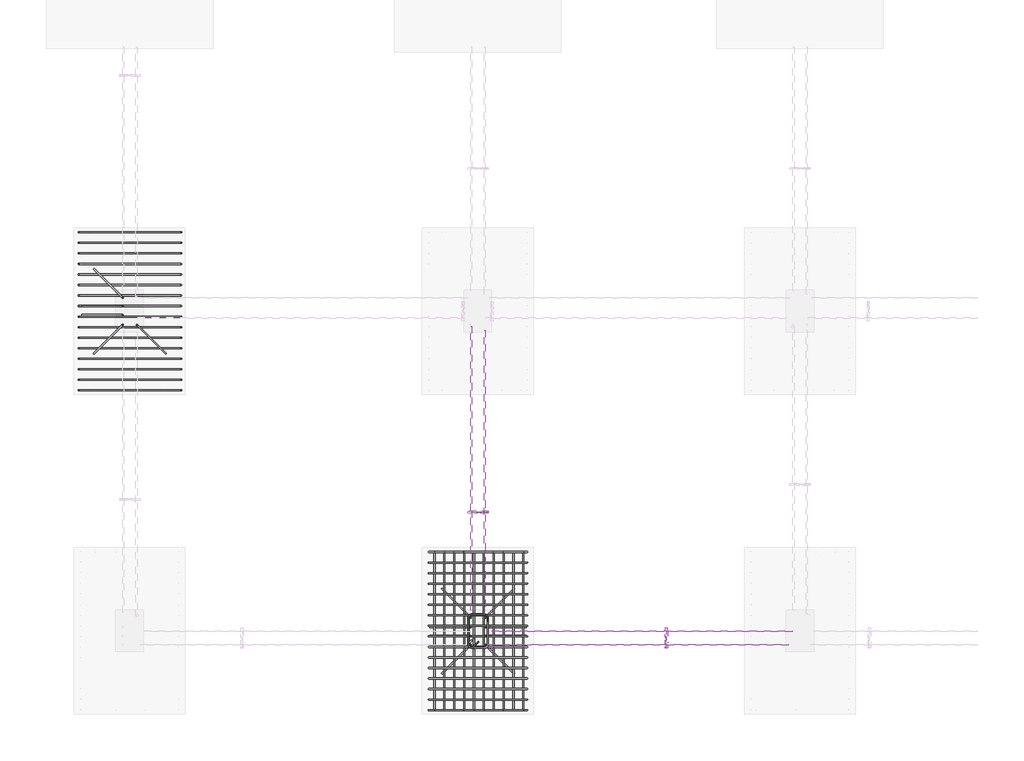
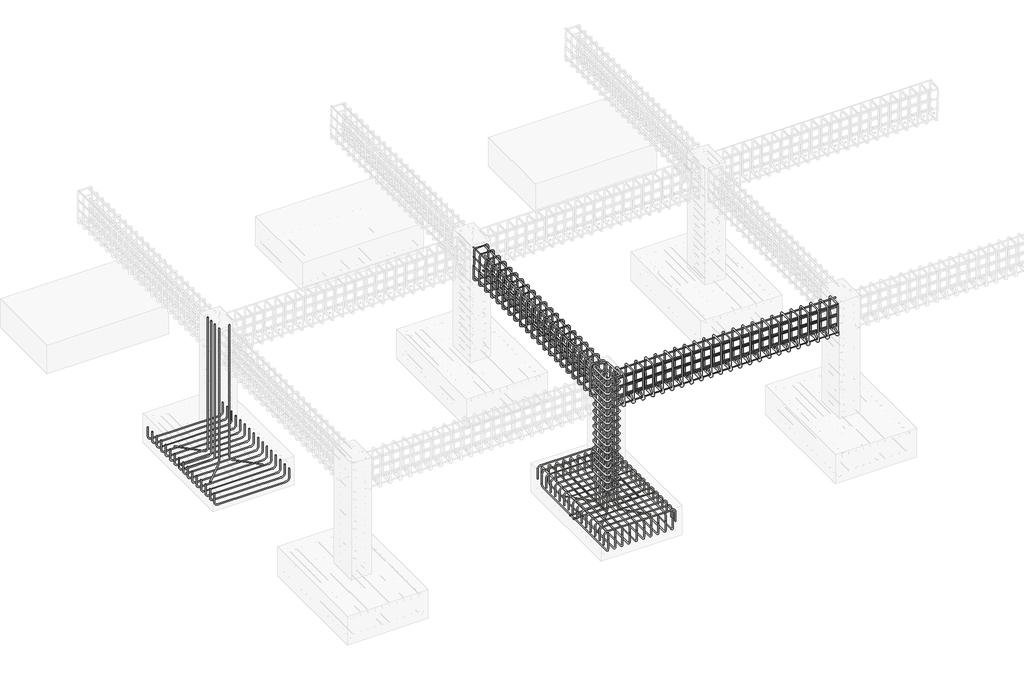
# One storey, part 3 of 20: 21 reinforcing bars.
"""IFC4 building model written with IfcOpenShell, lengths in millimetres."""

from ifc_helpers import new_model, si_unit, point, frame, origin, place, context, project, spatial, polyline, circle_curve, trimmed, segment, composite_curve, source, transform, mapped, element, save
from ifc_brep_helpers import swept_disk

model = new_model("IFC4")

# Units and contexts
model_context = context("Model", 3, world=origin())
ifc_project = project(units=[si_unit("LENGTHUNIT", "METRE", prefix="MILLI")], contexts=[model_context])

# Site, building, storey
site = spatial("IfcSite", under=ifc_project)
building = spatial("IfcBuilding", under=site)
storey = spatial("IfcBuildingStorey", under=building, Elevation=-1828.8)

# Reinforcing bars
placement = place(None, origin())
reinforcing_bar_shape = source(origin(), model_context, "Body", "SolidModel", [
    swept_disk(composite_curve([segment(polyline([(-5310.2912236, -1871.0168637, -2028.4704493), (-5310.2912236, -1871.0168637, -2175.7704493)]), True, "CONTINUOUS"), segment(trimmed(circle_curve(frame((-5356.6412236, -1871.0168637, -2175.7704493), z_axis=(0.0, 1.0, 0.0), x_axis=(46.349999999999454, 0.0, 0.0)), 46.35), [point((-5310.2912236, -1871.0168637, -2175.7704493))], [point((-5356.6412236, -1871.0168637, -2222.1204493))], True, "CARTESIAN"), True, "CONTINUOUS"), segment(polyline([(-5356.6412236, -1871.0168637, -2222.1204493), (-6371.2412236, -1871.0168637, -2222.1204493)]), True, "CONTINUOUS"), segment(trimmed(circle_curve(frame((-6371.2412236, -1871.0168637, -2175.7704493), z_axis=(0.0, 1.0, 0.0), x_axis=(0.0, 0.0, -46.34999999999991)), 46.35), [point((-6371.2412236, -1871.0168637, -2222.1204493))], [point((-6417.5912236, -1871.0168637, -2175.7704493))], True, "CARTESIAN"), True, "CONTINUOUS"), segment(polyline([(-6417.5912236, -1871.0168637, -2175.7704493), (-6417.5912236, -1871.0168637, -2028.4704493)]), True, "CONTINUOUS")], self_intersect=False), 6.35),
])
element("IfcReinforcingBar", 1, at=placement, inside=storey, context=model_context, shape_type="MappedRepresentation", body=[
    mapped(reinforcing_bar_shape, transform((0.0, 0.0, 0.0), x_axis=(1.0, 0.0, 0.0), y_axis=(0.0, 1.0, 0.0), z_axis=(0.0, 0.0, 1.0))),
    mapped(reinforcing_bar_shape, transform((0.0, -113.82, 0.0), x_axis=(1.0, 0.0, 0.0), y_axis=(0.0, 1.0, 0.0), z_axis=(0.0, 0.0, 1.0))),
    mapped(reinforcing_bar_shape, transform((0.0, -227.64, 0.0), x_axis=(1.0, 0.0, 0.0), y_axis=(0.0, 1.0, 0.0), z_axis=(0.0, 0.0, 1.0))),
    mapped(reinforcing_bar_shape, transform((0.0, -341.46, 0.0), x_axis=(1.0, 0.0, 0.0), y_axis=(0.0, 1.0, 0.0), z_axis=(0.0, 0.0, 1.0))),
    mapped(reinforcing_bar_shape, transform((0.0, -455.28, 0.0), x_axis=(1.0, 0.0, 0.0), y_axis=(0.0, 1.0, 0.0), z_axis=(0.0, 0.0, 1.0))),
    mapped(reinforcing_bar_shape, transform((0.0, -569.1, 0.0), x_axis=(1.0, 0.0, 0.0), y_axis=(0.0, 1.0, 0.0), z_axis=(0.0, 0.0, 1.0))),
    mapped(reinforcing_bar_shape, transform((0.0, -682.92, 0.0), x_axis=(1.0, 0.0, 0.0), y_axis=(0.0, 1.0, 0.0), z_axis=(0.0, 0.0, 1.0))),
    mapped(reinforcing_bar_shape, transform((0.0, -796.74, 0.0), x_axis=(1.0, 0.0, 0.0), y_axis=(0.0, 1.0, 0.0), z_axis=(0.0, 0.0, 1.0))),
    mapped(reinforcing_bar_shape, transform((0.0, -910.56, 0.0), x_axis=(1.0, 0.0, 0.0), y_axis=(0.0, 1.0, 0.0), z_axis=(0.0, 0.0, 1.0))),
    mapped(reinforcing_bar_shape, transform((0.0, -1024.38, 0.0), x_axis=(1.0, 0.0, 0.0), y_axis=(0.0, 1.0, 0.0), z_axis=(0.0, 0.0, 1.0))),
    mapped(reinforcing_bar_shape, transform((0.0, -1138.2, 0.0), x_axis=(1.0, 0.0, 0.0), y_axis=(0.0, 1.0, 0.0), z_axis=(0.0, 0.0, 1.0))),
    mapped(reinforcing_bar_shape, transform((0.0, -1252.02, 0.0), x_axis=(1.0, 0.0, 0.0), y_axis=(0.0, 1.0, 0.0), z_axis=(0.0, 0.0, 1.0))),
    mapped(reinforcing_bar_shape, transform((0.0, -1365.84, 0.0), x_axis=(1.0, 0.0, 0.0), y_axis=(0.0, 1.0, 0.0), z_axis=(0.0, 0.0, 1.0))),
    mapped(reinforcing_bar_shape, transform((0.0, -1479.66, 0.0), x_axis=(1.0, 0.0, 0.0), y_axis=(0.0, 1.0, 0.0), z_axis=(0.0, 0.0, 1.0))),
    mapped(reinforcing_bar_shape, transform((0.0, -1593.48, 0.0), x_axis=(1.0, 0.0, 0.0), y_axis=(0.0, 1.0, 0.0), z_axis=(0.0, 0.0, 1.0))),
    mapped(reinforcing_bar_shape, transform((0.0, -1707.3, 0.0), x_axis=(1.0, 0.0, 0.0), y_axis=(0.0, 1.0, 0.0), z_axis=(0.0, 0.0, 1.0))),
])
reinforcing_bar_2_shape = source(origin(), model_context, "Body", "SolidModel", [
    swept_disk(composite_curve([segment(polyline([(-1573.3103556, -7032.7168637, -2068.8), (-1573.3103556, -7032.7168637, -1921.5)]), True, "CONTINUOUS"), segment(trimmed(circle_curve(frame((-1619.6603556, -7032.7168637, -1921.5), z_axis=(0.0, -1.0, 0.0), x_axis=(46.34999999999991, 0.0, 0.0)), 46.35), [point((-1573.3103556, -7032.7168637, -1921.5))], [point((-1619.6603556, -7032.7168637, -1875.15))], True, "CARTESIAN"), True, "CONTINUOUS"), segment(polyline([(-1619.6603556, -7032.7168637, -1875.15), (-2587.3817473, -7032.7168637, -1875.15)]), True, "CONTINUOUS"), segment(trimmed(circle_curve(frame((-2587.3817473, -7032.7168637, -1921.5), z_axis=(0.0, -1.0, 0.0), x_axis=(0.0, 0.0, 46.34999999999991)), 46.35), [point((-2587.3817473, -7032.7168637, -1875.15))], [point((-2633.7317473, -7032.7168637, -1921.5))], True, "CARTESIAN"), True, "CONTINUOUS"), segment(polyline([(-2633.7317473, -7032.7168637, -1921.5), (-2633.7317473, -7032.7168637, -2068.8)]), True, "CONTINUOUS")], self_intersect=False), 6.35),
])
element("IfcReinforcingBar", 2, at=placement, inside=storey, context=model_context, shape_type="MappedRepresentation", body=[
    mapped(reinforcing_bar_2_shape, transform((0.0, 0.0, 0.0), x_axis=(1.0, 0.0, 0.0), y_axis=(0.0, 1.0, 0.0), z_axis=(0.0, 0.0, 1.0))),
    mapped(reinforcing_bar_2_shape, transform((0.0, 113.82, 0.0), x_axis=(1.0, 0.0, 0.0), y_axis=(0.0, 1.0, 0.0), z_axis=(0.0, 0.0, 1.0))),
    mapped(reinforcing_bar_2_shape, transform((0.0, 227.64, 0.0), x_axis=(1.0, 0.0, 0.0), y_axis=(0.0, 1.0, 0.0), z_axis=(0.0, 0.0, 1.0))),
    mapped(reinforcing_bar_2_shape, transform((0.0, 341.46, 0.0), x_axis=(1.0, 0.0, 0.0), y_axis=(0.0, 1.0, 0.0), z_axis=(0.0, 0.0, 1.0))),
    mapped(reinforcing_bar_2_shape, transform((0.0, 455.28, 0.0), x_axis=(1.0, 0.0, 0.0), y_axis=(0.0, 1.0, 0.0), z_axis=(0.0, 0.0, 1.0))),
    mapped(reinforcing_bar_2_shape, transform((0.0, 569.1, 0.0), x_axis=(1.0, 0.0, 0.0), y_axis=(0.0, 1.0, 0.0), z_axis=(0.0, 0.0, 1.0))),
    mapped(reinforcing_bar_2_shape, transform((0.0, 682.92, 0.0), x_axis=(1.0, 0.0, 0.0), y_axis=(0.0, 1.0, 0.0), z_axis=(0.0, 0.0, 1.0))),
    mapped(reinforcing_bar_2_shape, transform((0.0, 796.74, 0.0), x_axis=(1.0, 0.0, 0.0), y_axis=(0.0, 1.0, 0.0), z_axis=(0.0, 0.0, 1.0))),
    mapped(reinforcing_bar_2_shape, transform((0.0, 910.56, 0.0), x_axis=(1.0, 0.0, 0.0), y_axis=(0.0, 1.0, 0.0), z_axis=(0.0, 0.0, 1.0))),
    mapped(reinforcing_bar_2_shape, transform((0.0, 1024.38, 0.0), x_axis=(1.0, 0.0, 0.0), y_axis=(0.0, 1.0, 0.0), z_axis=(0.0, 0.0, 1.0))),
    mapped(reinforcing_bar_2_shape, transform((0.0, 1138.2, 0.0), x_axis=(1.0, 0.0, 0.0), y_axis=(0.0, 1.0, 0.0), z_axis=(0.0, 0.0, 1.0))),
    mapped(reinforcing_bar_2_shape, transform((0.0, 1252.02, 0.0), x_axis=(1.0, 0.0, 0.0), y_axis=(0.0, 1.0, 0.0), z_axis=(0.0, 0.0, 1.0))),
    mapped(reinforcing_bar_2_shape, transform((0.0, 1365.84, 0.0), x_axis=(1.0, 0.0, 0.0), y_axis=(0.0, 1.0, 0.0), z_axis=(0.0, 0.0, 1.0))),
    mapped(reinforcing_bar_2_shape, transform((0.0, 1479.66, 0.0), x_axis=(1.0, 0.0, 0.0), y_axis=(0.0, 1.0, 0.0), z_axis=(0.0, 0.0, 1.0))),
    mapped(reinforcing_bar_2_shape, transform((0.0, 1593.48, 0.0), x_axis=(1.0, 0.0, 0.0), y_axis=(0.0, 1.0, 0.0), z_axis=(0.0, 0.0, 1.0))),
    mapped(reinforcing_bar_2_shape, transform((0.0, 1707.3, 0.0), x_axis=(1.0, 0.0, 0.0), y_axis=(0.0, 1.0, 0.0), z_axis=(0.0, 0.0, 1.0))),
])
reinforcing_bar_3_shape = source(origin(), model_context, "Body", "SolidModel", [
    swept_disk(composite_curve([segment(polyline([(-1612.8777058, -7032.7168637, -2008.6504502), (-1612.8777058, -7032.7168637, -2155.9504502)]), True, "CONTINUOUS"), segment(trimmed(circle_curve(frame((-1612.8777058, -6986.3668637, -2155.9504502), z_axis=(1.0, 0.0, 0.0), x_axis=(0.0, -46.350000000000364, 0.0)), 46.35), [point((-1612.8777058, -7032.7168637, -2155.9504502))], [point((-1612.8777058, -6986.3668637, -2202.3004502))], True, "CARTESIAN"), True, "CONTINUOUS"), segment(polyline([(-1612.8777058, -6986.3668637, -2202.3004502), (-1612.8777058, -5371.7668637, -2202.3004502)]), True, "CONTINUOUS"), segment(trimmed(circle_curve(frame((-1612.8777058, -5371.7668637, -2155.9504502), z_axis=(1.0, 0.0, 0.0), x_axis=(0.0, 0.0, -46.34999999999991)), 46.35), [point((-1612.8777058, -5371.7668637, -2202.3004502))], [point((-1612.8777058, -5325.4168637, -2155.9504502))], True, "CARTESIAN"), True, "CONTINUOUS"), segment(polyline([(-1612.8777058, -5325.4168637, -2155.9504502), (-1612.8777058, -5325.4168637, -2008.6504502)]), True, "CONTINUOUS")], self_intersect=False), 6.35),
])
element("IfcReinforcingBar", 3, at=placement, inside=storey, context=model_context, shape_type="MappedRepresentation", body=[
    mapped(reinforcing_bar_3_shape, transform((0.0, 0.0, 0.0), x_axis=(1.0, 0.0, 0.0), y_axis=(0.0, 1.0, 0.0), z_axis=(0.0, 0.0, 1.0))),
    mapped(reinforcing_bar_3_shape, transform((-106.7711398, 0.0, 0.0), x_axis=(1.0, 0.0, 0.0), y_axis=(0.0, 1.0, 0.0), z_axis=(0.0, 0.0, 1.0))),
    mapped(reinforcing_bar_3_shape, transform((-213.5422797, 0.0, 0.0), x_axis=(1.0, 0.0, 0.0), y_axis=(0.0, 1.0, 0.0), z_axis=(0.0, 0.0, 1.0))),
    mapped(reinforcing_bar_3_shape, transform((-320.3134195, 0.0, 0.0), x_axis=(1.0, 0.0, 0.0), y_axis=(0.0, 1.0, 0.0), z_axis=(0.0, 0.0, 1.0))),
    mapped(reinforcing_bar_3_shape, transform((-427.0845593, 0.0, 0.0), x_axis=(1.0, 0.0, 0.0), y_axis=(0.0, 1.0, 0.0), z_axis=(0.0, 0.0, 1.0))),
    mapped(reinforcing_bar_3_shape, transform((-533.8556992, 0.0, 0.0), x_axis=(1.0, 0.0, 0.0), y_axis=(0.0, 1.0, 0.0), z_axis=(0.0, 0.0, 1.0))),
    mapped(reinforcing_bar_3_shape, transform((-640.626839, 0.0, 0.0), x_axis=(1.0, 0.0, 0.0), y_axis=(0.0, 1.0, 0.0), z_axis=(0.0, 0.0, 1.0))),
    mapped(reinforcing_bar_3_shape, transform((-747.3979788, 0.0, 0.0), x_axis=(1.0, 0.0, 0.0), y_axis=(0.0, 1.0, 0.0), z_axis=(0.0, 0.0, 1.0))),
    mapped(reinforcing_bar_3_shape, transform((-854.1691187, 0.0, 0.0), x_axis=(1.0, 0.0, 0.0), y_axis=(0.0, 1.0, 0.0), z_axis=(0.0, 0.0, 1.0))),
    mapped(reinforcing_bar_3_shape, transform((-960.9402585, 0.0, 0.0), x_axis=(1.0, 0.0, 0.0), y_axis=(0.0, 1.0, 0.0), z_axis=(0.0, 0.0, 1.0))),
])
reinforcing_bar_4_shape = source(origin(), model_context, "Body", "SolidModel", [
    swept_disk(composite_curve([segment(polyline([(-2573.8179643, -7032.7168637, -2088.5147466), (-2573.8179643, -7032.7168637, -1941.2147466)]), True, "CONTINUOUS"), segment(trimmed(circle_curve(frame((-2573.8179643, -6986.3668637, -1941.2147466), z_axis=(-1.0, 0.0, 0.0), x_axis=(0.0, -46.350000000000364, 0.0)), 46.35), [point((-2573.8179643, -7032.7168637, -1941.2147466))], [point((-2573.8179643, -6986.3668637, -1894.8647466))], True, "CARTESIAN"), True, "CONTINUOUS"), segment(polyline([(-2573.8179643, -6986.3668637, -1894.8647466), (-2573.8179643, -5371.7668637, -1894.8647466)]), True, "CONTINUOUS"), segment(trimmed(circle_curve(frame((-2573.8179643, -5371.7668637, -1941.2147466), z_axis=(-1.0, 0.0, 0.0), x_axis=(0.0, 0.0, 46.34999999999991)), 46.35), [point((-2573.8179643, -5371.7668637, -1894.8647466))], [point((-2573.8179643, -5325.4168637, -1941.2147466))], True, "CARTESIAN"), True, "CONTINUOUS"), segment(polyline([(-2573.8179643, -5325.4168637, -1941.2147466), (-2573.8179643, -5325.4168637, -2088.5147466)]), True, "CONTINUOUS")], self_intersect=False), 6.35),
])
element("IfcReinforcingBar", 4, at=placement, inside=storey, context=model_context, shape_type="MappedRepresentation", body=[
    mapped(reinforcing_bar_4_shape, transform((0.0, 0.0, 0.0), x_axis=(1.0, 0.0, 0.0), y_axis=(0.0, 1.0, 0.0), z_axis=(0.0, 0.0, 1.0))),
    mapped(reinforcing_bar_4_shape, transform((106.7711398, 0.0, 0.0), x_axis=(1.0, 0.0, 0.0), y_axis=(0.0, 1.0, 0.0), z_axis=(0.0, 0.0, 1.0))),
    mapped(reinforcing_bar_4_shape, transform((213.5422797, 0.0, 0.0), x_axis=(1.0, 0.0, 0.0), y_axis=(0.0, 1.0, 0.0), z_axis=(0.0, 0.0, 1.0))),
    mapped(reinforcing_bar_4_shape, transform((320.3134195, 0.0, 0.0), x_axis=(1.0, 0.0, 0.0), y_axis=(0.0, 1.0, 0.0), z_axis=(0.0, 0.0, 1.0))),
    mapped(reinforcing_bar_4_shape, transform((427.0845593, 0.0, 0.0), x_axis=(1.0, 0.0, 0.0), y_axis=(0.0, 1.0, 0.0), z_axis=(0.0, 0.0, 1.0))),
    mapped(reinforcing_bar_4_shape, transform((533.8556992, 0.0, 0.0), x_axis=(1.0, 0.0, 0.0), y_axis=(0.0, 1.0, 0.0), z_axis=(0.0, 0.0, 1.0))),
    mapped(reinforcing_bar_4_shape, transform((640.626839, 0.0, 0.0), x_axis=(1.0, 0.0, 0.0), y_axis=(0.0, 1.0, 0.0), z_axis=(0.0, 0.0, 1.0))),
    mapped(reinforcing_bar_4_shape, transform((747.3979788, 0.0, 0.0), x_axis=(1.0, 0.0, 0.0), y_axis=(0.0, 1.0, 0.0), z_axis=(0.0, 0.0, 1.0))),
    mapped(reinforcing_bar_4_shape, transform((854.1691187, 0.0, 0.0), x_axis=(1.0, 0.0, 0.0), y_axis=(0.0, 1.0, 0.0), z_axis=(0.0, 0.0, 1.0))),
    mapped(reinforcing_bar_4_shape, transform((960.9402585, 0.0, 0.0), x_axis=(1.0, 0.0, 0.0), y_axis=(0.0, 1.0, 0.0), z_axis=(0.0, 0.0, 1.0))),
])
reinforcing_bar_5_shape = source(origin(), model_context, "Body", "SolidModel", [
    swept_disk(composite_curve([segment(polyline([(-6384.4701101, -2670.9908411, -2151.8747939), (-5987.4527787, -2670.9908411, -2151.8747939)]), True, "CONTINUOUS"), segment(trimmed(circle_curve(frame((-5987.4527787, -2670.9908411, -2105.5247939), z_axis=(0.0, -1.0, 0.0), x_axis=(0.0, 0.0, -46.34999999999991)), 46.35), [point((-5987.4527787, -2670.9908411, -2151.8747939))], [point((-5941.1027787, -2670.9908411, -2105.5247939))], True, "CARTESIAN"), True, "CONTINUOUS"), segment(polyline([(-5941.1027787, -2670.9908411, -2105.5247939), (-5941.1027787, -2670.9908411, -40.0)]), True, "CONTINUOUS")], self_intersect=False), 6.35),
])
element("IfcReinforcingBar", 5, at=placement, inside=storey, context=model_context, shape_type="MappedRepresentation", body=[
    mapped(reinforcing_bar_5_shape, transform((0.0, 0.0, 0.0), x_axis=(1.0, 0.0, 0.0), y_axis=(0.0, 1.0, 0.0), z_axis=(0.0, 0.0, 1.0))),
    mapped(reinforcing_bar_5_shape, transform((0.0, -93.9182821, 0.0), x_axis=(1.0, 0.0, 0.0), y_axis=(0.0, 1.0, 0.0), z_axis=(0.0, 0.0, 1.0))),
])
element("IfcReinforcingBar", 6, at=placement, inside=storey, context=model_context, shape_type="SolidModel", body=[
    swept_disk(composite_curve([segment(polyline([(-6254.6108252, -3184.1708088, -2151.8747939), (-5973.877178, -2903.4371615, -2151.8747939)]), True, "CONTINUOUS"), segment(trimmed(circle_curve(frame((-5973.877178, -2903.4371615, -2105.5247939), z_axis=(0.7071067811865442, -0.7071067811865509, 0.0), x_axis=(0.0, 0.0, -46.34999999999991)), 46.35), [point((-5973.877178, -2903.4371615, -2151.8747939))], [point((-5941.1027787, -2870.6627622, -2105.5247939))], True, "CARTESIAN"), True, "CONTINUOUS"), segment(polyline([(-5941.1027787, -2870.6627622, -2105.5247939), (-5941.1027787, -2870.6627622, -40.0)]), True, "CONTINUOUS")], self_intersect=False), 6.35),
])
element("IfcReinforcingBar", 7, at=placement, inside=storey, context=model_context, shape_type="SolidModel", body=[
    swept_disk(composite_curve([segment(polyline([(-5473.271622, -3184.1708088, -2151.8747939), (-5754.0052693, -2903.4371615, -2151.8747939)]), True, "CONTINUOUS"), segment(trimmed(circle_curve(frame((-5754.0052693, -2903.4371615, -2105.5247939), z_axis=(0.7071067811865442, 0.7071067811865509, 0.0), x_axis=(0.0, 0.0, -46.34999999999991)), 46.35), [point((-5754.0052693, -2903.4371615, -2151.8747939))], [point((-5786.7796686, -2870.6627622, -2105.5247939))], True, "CARTESIAN"), True, "CONTINUOUS"), segment(polyline([(-5786.7796686, -2870.6627622, -2105.5247939), (-5786.7796686, -2870.6627622, -40.0)]), True, "CONTINUOUS")], self_intersect=False), 6.35),
])
element("IfcReinforcingBar", 8, at=placement, inside=storey, context=model_context, shape_type="SolidModel", body=[
    swept_disk(composite_curve([segment(polyline([(-6254.6108252, -2265.1629186, -2151.8747939), (-5973.877178, -2545.8965659, -2151.8747939)]), True, "CONTINUOUS"), segment(trimmed(circle_curve(frame((-5973.877178, -2545.8965659, -2105.5247939), z_axis=(-0.7071067811865442, -0.7071067811865509, 0.0), x_axis=(0.0, 0.0, -46.34999999999991)), 46.35), [point((-5973.877178, -2545.8965659, -2151.8747939))], [point((-5941.1027787, -2578.6709652, -2105.5247939))], True, "CARTESIAN"), True, "CONTINUOUS"), segment(polyline([(-5941.1027787, -2578.6709652, -2105.5247939), (-5941.1027787, -2578.6709652, -40.0)]), True, "CONTINUOUS")], self_intersect=False), 6.35),
])
reinforcing_bar_6_shape = source(origin(), model_context, "Body", "SolidModel", [
    swept_disk(composite_curve([segment(polyline([(-2097.1746502, -6292.7910983, -46.35), (-2152.9182131, -6348.5346613, -46.35)]), True, "CONTINUOUS"), segment(trimmed(circle_curve(frame((-2175.0860107, -6326.3668637, -46.35), z_axis=(0.0, 0.0, -1.0), x_axis=(22.167797600000085, -22.167797600000085, 0.0)), 31.35), [point((-2152.9182131, -6348.5346613, -46.35))], [point((-2206.4360107, -6326.3668637, -46.35))], True, "CARTESIAN"), True, "CONTINUOUS"), segment(polyline([(-2206.4360107, -6326.3668637, -46.35), (-2206.4360107, -6031.7668637, -46.35)]), True, "CONTINUOUS"), segment(trimmed(circle_curve(frame((-2175.0860107, -6031.7668637, -46.35), z_axis=(0.0, 0.0, -1.0), x_axis=(-31.350000000000364, 0.0, 0.0)), 31.35), [point((-2206.4360107, -6031.7668637, -46.35))], [point((-2175.0860107, -6000.4168637, -46.35))], True, "CARTESIAN"), True, "CONTINUOUS"), segment(polyline([(-2175.0860107, -6000.4168637, -46.35), (-2030.4860107, -6000.4168637, -46.35)]), True, "CONTINUOUS"), segment(trimmed(circle_curve(frame((-2030.4860107, -6031.7470786, -45.2363875), z_axis=(0.0, -0.035521928334481916, -0.9993688971583016), x_axis=(0.0, 31.3302149000001, -1.1136125000000021)), 31.35), [point((-2030.4860107, -6000.4168637, -46.35))], [point((-1999.1360107, -6031.7470786, -45.2363875))], True, "CARTESIAN"), True, "CONTINUOUS"), segment(polyline([(-1999.1360107, -6031.7470786, -45.2363875), (-1999.1360107, -6326.3866488, -34.7636125)]), True, "CONTINUOUS"), segment(trimmed(circle_curve(frame((-2030.4860107, -6326.3866488, -34.7636125), z_axis=(0.0, -0.035521928334481916, -0.9993688971583016), x_axis=(31.34999999999991, 0.0, 0.0)), 31.35), [point((-1999.1360107, -6326.3866488, -34.7636125))], [point((-2030.4860107, -6357.7168637, -33.65))], True, "CARTESIAN"), True, "CONTINUOUS"), segment(polyline([(-2030.4860107, -6357.7168637, -33.65), (-2175.0860107, -6357.7168637, -33.65)]), True, "CONTINUOUS"), segment(trimmed(circle_curve(frame((-2175.0860107, -6326.3668637, -33.65), z_axis=(0.0, 0.0, -1.0), x_axis=(0.0, -31.350000000000364, 0.0)), 31.35), [point((-2175.0860107, -6357.7168637, -33.65))], [point((-2197.2538083, -6304.1990661, -33.65))], True, "CARTESIAN"), True, "CONTINUOUS"), segment(polyline([(-2197.2538083, -6304.1990661, -33.65), (-2141.5102453, -6248.4555031, -33.65)]), True, "CONTINUOUS")], self_intersect=False), 6.35),
])
element("IfcReinforcingBar", 9, at=placement, inside=storey, context=model_context, shape_type="MappedRepresentation", body=[
    mapped(reinforcing_bar_6_shape, transform((0.0, 0.0, 0.0), x_axis=(1.0, 0.0, 0.0), y_axis=(0.0, 1.0, 0.0), z_axis=(0.0, 0.0, 1.0))),
    mapped(reinforcing_bar_6_shape, transform((0.0, 0.0, -115.74), x_axis=(1.0, 0.0, 0.0), y_axis=(0.0, 1.0, 0.0), z_axis=(0.0, 0.0, 1.0))),
    mapped(reinforcing_bar_6_shape, transform((0.0, 0.0, -231.48), x_axis=(1.0, 0.0, 0.0), y_axis=(0.0, 1.0, 0.0), z_axis=(0.0, 0.0, 1.0))),
    mapped(reinforcing_bar_6_shape, transform((0.0, 0.0, -347.22), x_axis=(1.0, 0.0, 0.0), y_axis=(0.0, 1.0, 0.0), z_axis=(0.0, 0.0, 1.0))),
    mapped(reinforcing_bar_6_shape, transform((0.0, 0.0, -462.96), x_axis=(1.0, 0.0, 0.0), y_axis=(0.0, 1.0, 0.0), z_axis=(0.0, 0.0, 1.0))),
    mapped(reinforcing_bar_6_shape, transform((0.0, 0.0, -578.7), x_axis=(1.0, 0.0, 0.0), y_axis=(0.0, 1.0, 0.0), z_axis=(0.0, 0.0, 1.0))),
    mapped(reinforcing_bar_6_shape, transform((0.0, 0.0, -694.44), x_axis=(1.0, 0.0, 0.0), y_axis=(0.0, 1.0, 0.0), z_axis=(0.0, 0.0, 1.0))),
    mapped(reinforcing_bar_6_shape, transform((0.0, 0.0, -810.18), x_axis=(1.0, 0.0, 0.0), y_axis=(0.0, 1.0, 0.0), z_axis=(0.0, 0.0, 1.0))),
    mapped(reinforcing_bar_6_shape, transform((0.0, 0.0, -925.92), x_axis=(1.0, 0.0, 0.0), y_axis=(0.0, 1.0, 0.0), z_axis=(0.0, 0.0, 1.0))),
    mapped(reinforcing_bar_6_shape, transform((0.0, 0.0, -1041.66), x_axis=(1.0, 0.0, 0.0), y_axis=(0.0, 1.0, 0.0), z_axis=(0.0, 0.0, 1.0))),
    mapped(reinforcing_bar_6_shape, transform((0.0, 0.0, -1157.4), x_axis=(1.0, 0.0, 0.0), y_axis=(0.0, 1.0, 0.0), z_axis=(0.0, 0.0, 1.0))),
    mapped(reinforcing_bar_6_shape, transform((0.0, 0.0, -1273.14), x_axis=(1.0, 0.0, 0.0), y_axis=(0.0, 1.0, 0.0), z_axis=(0.0, 0.0, 1.0))),
    mapped(reinforcing_bar_6_shape, transform((0.0, 0.0, -1388.88), x_axis=(1.0, 0.0, 0.0), y_axis=(0.0, 1.0, 0.0), z_axis=(0.0, 0.0, 1.0))),
    mapped(reinforcing_bar_6_shape, transform((0.0, 0.0, -1504.62), x_axis=(1.0, 0.0, 0.0), y_axis=(0.0, 1.0, 0.0), z_axis=(0.0, 0.0, 1.0))),
    mapped(reinforcing_bar_6_shape, transform((0.0, 0.0, -1620.36), x_axis=(1.0, 0.0, 0.0), y_axis=(0.0, 1.0, 0.0), z_axis=(0.0, 0.0, 1.0))),
    mapped(reinforcing_bar_6_shape, transform((0.0, 0.0, -1736.1), x_axis=(1.0, 0.0, 0.0), y_axis=(0.0, 1.0, 0.0), z_axis=(0.0, 0.0, 1.0))),
])
reinforcing_bar_7_shape = source(origin(), model_context, "Body", "SolidModel", [
    swept_disk(composite_curve([segment(polyline([(-1582.2571243, -6232.7428863, -2151.8747939), (-1979.2744557, -6232.7428863, -2151.8747939)]), True, "CONTINUOUS"), segment(trimmed(circle_curve(frame((-1979.2744557, -6232.7428863, -2105.5247939), z_axis=(0.0, 1.0, 0.0), x_axis=(0.0, 0.0, -46.34999999999991)), 46.35), [point((-1979.2744557, -6232.7428863, -2151.8747939))], [point((-2025.6244557, -6232.7428863, -2105.5247939))], True, "CARTESIAN"), True, "CONTINUOUS"), segment(polyline([(-2025.6244557, -6232.7428863, -2105.5247939), (-2025.6244557, -6232.7428863, -40.0)]), True, "CONTINUOUS")], self_intersect=False), 6.35),
])
element("IfcReinforcingBar", 10, at=placement, inside=storey, context=model_context, shape_type="MappedRepresentation", body=[
    mapped(reinforcing_bar_7_shape, transform((0.0, 0.0, 0.0), x_axis=(1.0, 0.0, 0.0), y_axis=(0.0, 1.0, 0.0), z_axis=(0.0, 0.0, 1.0))),
    mapped(reinforcing_bar_7_shape, transform((0.0, 93.9182821, 0.0), x_axis=(1.0, 0.0, 0.0), y_axis=(0.0, 1.0, 0.0), z_axis=(0.0, 0.0, 1.0))),
])
element("IfcReinforcingBar", 11, at=placement, inside=storey, context=model_context, shape_type="SolidModel", body=[
    swept_disk(composite_curve([segment(polyline([(-1712.1164091, -5719.5629186, -2151.8747939), (-1992.8500564, -6000.2965659, -2151.8747939)]), True, "CONTINUOUS"), segment(trimmed(circle_curve(frame((-1992.8500564, -6000.2965659, -2105.5247939), z_axis=(-0.7071067811865442, 0.7071067811865509, 0.0), x_axis=(0.0, 0.0, -46.34999999999991)), 46.35), [point((-1992.8500564, -6000.2965659, -2151.8747939))], [point((-2025.6244557, -6033.0709652, -2105.5247939))], True, "CARTESIAN"), True, "CONTINUOUS"), segment(polyline([(-2025.6244557, -6033.0709652, -2105.5247939), (-2025.6244557, -6033.0709652, -40.0)]), True, "CONTINUOUS")], self_intersect=False), 6.35),
])
element("IfcReinforcingBar", 12, at=placement, inside=storey, context=model_context, shape_type="SolidModel", body=[
    swept_disk(composite_curve([segment(polyline([(-2493.4556123, -5719.5629186, -2151.8747939), (-2212.721965, -6000.2965659, -2151.8747939)]), True, "CONTINUOUS"), segment(trimmed(circle_curve(frame((-2212.721965, -6000.2965659, -2105.5247939), z_axis=(-0.7071067811865442, -0.7071067811865509, 0.0), x_axis=(0.0, 0.0, -46.34999999999991)), 46.35), [point((-2212.721965, -6000.2965659, -2151.8747939))], [point((-2179.9475657, -6033.0709652, -2105.5247939))], True, "CARTESIAN"), True, "CONTINUOUS"), segment(polyline([(-2179.9475657, -6033.0709652, -2105.5247939), (-2179.9475657, -6033.0709652, -40.0)]), True, "CONTINUOUS")], self_intersect=False), 6.35),
])
element("IfcReinforcingBar", 13, at=placement, inside=storey, context=model_context, shape_type="SolidModel", body=[
    swept_disk(composite_curve([segment(polyline([(-1712.1164091, -6638.5708088, -2151.8747939), (-1992.8500564, -6357.8371615, -2151.8747939)]), True, "CONTINUOUS"), segment(trimmed(circle_curve(frame((-1992.8500564, -6357.8371615, -2105.5247939), z_axis=(0.7071067811865442, 0.7071067811865509, 0.0), x_axis=(0.0, 0.0, -46.34999999999991)), 46.35), [point((-1992.8500564, -6357.8371615, -2151.8747939))], [point((-2025.6244557, -6325.0627622, -2105.5247939))], True, "CARTESIAN"), True, "CONTINUOUS"), segment(polyline([(-2025.6244557, -6325.0627622, -2105.5247939), (-2025.6244557, -6325.0627622, -40.0)]), True, "CONTINUOUS")], self_intersect=False), 6.35),
])
element("IfcReinforcingBar", 14, at=placement, inside=storey, context=model_context, shape_type="SolidModel", body=[
    swept_disk(composite_curve([segment(polyline([(-2493.4556123, -6638.5708088, -2151.8747939), (-2212.721965, -6357.8371615, -2151.8747939)]), True, "CONTINUOUS"), segment(trimmed(circle_curve(frame((-2212.721965, -6357.8371615, -2105.5247939), z_axis=(0.7071067811865442, -0.7071067811865509, 0.0), x_axis=(0.0, 0.0, -46.34999999999991)), 46.35), [point((-2212.721965, -6357.8371615, -2151.8747939))], [point((-2179.9475657, -6325.0627622, -2105.5247939))], True, "CARTESIAN"), True, "CONTINUOUS"), segment(polyline([(-2179.9475657, -6325.0627622, -2105.5247939), (-2179.9475657, -6325.0627622, -40.0)]), True, "CONTINUOUS")], self_intersect=False), 6.35),
])
reinforcing_bar_8_shape = source(origin(), model_context, "Body", "SolidModel", [
    swept_disk(composite_curve([segment(polyline([(-2623.3148971, -6232.7428863, -2151.8747939), (-2226.2975657, -6232.7428863, -2151.8747939)]), True, "CONTINUOUS"), segment(trimmed(circle_curve(frame((-2226.2975657, -6232.7428863, -2105.5247939), z_axis=(0.0, -1.0, 0.0), x_axis=(0.0, 0.0, -46.34999999999991)), 46.35), [point((-2226.2975657, -6232.7428863, -2151.8747939))], [point((-2179.9475657, -6232.7428863, -2105.5247939))], True, "CARTESIAN"), True, "CONTINUOUS"), segment(polyline([(-2179.9475657, -6232.7428863, -2105.5247939), (-2179.9475657, -6232.7428863, -40.0)]), True, "CONTINUOUS")], self_intersect=False), 6.35),
])
element("IfcReinforcingBar", 15, at=placement, inside=storey, context=model_context, shape_type="MappedRepresentation", body=[
    mapped(reinforcing_bar_8_shape, transform((0.0, 0.0, 0.0), x_axis=(1.0, 0.0, 0.0), y_axis=(0.0, 1.0, 0.0), z_axis=(0.0, 0.0, 1.0))),
    mapped(reinforcing_bar_8_shape, transform((0.0, 93.9182821, 0.0), x_axis=(1.0, 0.0, 0.0), y_axis=(0.0, 1.0, 0.0), z_axis=(0.0, 0.0, 1.0))),
])
reinforcing_bar_9_shape = source(origin(), model_context, "Body", "SolidModel", [
    swept_disk(composite_curve([segment(polyline([(-2108.3973712, -2956.0168637, -488.7242346), (-2052.6538083, -2956.0168637, -544.4677976)]), True, "CONTINUOUS"), segment(trimmed(circle_curve(frame((-2030.4860107, -2956.0168637, -522.3), z_axis=(0.0, -1.0, 0.0), x_axis=(-22.167797600000085, 0.0, -22.167797600000085)), 31.35), [point((-2052.6538083, -2956.0168637, -544.4677976))], [point((-1999.1360107, -2956.0168637, -522.3))], True, "CARTESIAN"), True, "CONTINUOUS"), segment(polyline([(-1999.1360107, -2956.0168637, -522.3), (-1999.1360107, -2956.0168637, -77.7)]), True, "CONTINUOUS"), segment(trimmed(circle_curve(frame((-2030.4860107, -2956.0168637, -77.7), z_axis=(0.0, -1.0, 0.0), x_axis=(31.34999999999991, 0.0, 0.0)), 31.35), [point((-1999.1360107, -2956.0168637, -77.7))], [point((-2030.4860107, -2956.0168637, -46.35))], True, "CARTESIAN"), True, "CONTINUOUS"), segment(polyline([(-2030.4860107, -2956.0168637, -46.35), (-2175.0860107, -2956.0168637, -46.35)]), True, "CONTINUOUS"), segment(trimmed(circle_curve(frame((-2175.0860107, -2955.232278, -77.6901807), z_axis=(0.0, -0.9996867842138424, -0.025026655153786322), x_axis=(0.0, -0.784585700000207, 31.340180699999998)), 31.35), [point((-2175.0860107, -2956.0168637, -46.35))], [point((-2206.4360107, -2955.232278, -77.6901807))], True, "CARTESIAN"), True, "CONTINUOUS"), segment(polyline([(-2206.4360107, -2955.232278, -77.6901807), (-2206.4360107, -2944.1014493, -522.3098193)]), True, "CONTINUOUS"), segment(trimmed(circle_curve(frame((-2175.0860107, -2944.1014493, -522.3098193), z_axis=(0.0, -0.9996867842138424, -0.025026655153786322), x_axis=(-31.350000000000364, 0.0, 0.0)), 31.35), [point((-2206.4360107, -2944.1014493, -522.3098193))], [point((-2175.0860107, -2943.3168637, -553.65))], True, "CARTESIAN"), True, "CONTINUOUS"), segment(polyline([(-2175.0860107, -2943.3168637, -553.65), (-2030.4860107, -2943.3168637, -553.65)]), True, "CONTINUOUS"), segment(trimmed(circle_curve(frame((-2030.4860107, -2943.3168637, -522.3), z_axis=(0.0, -1.0, 0.0), x_axis=(0.0, 0.0, -31.350000000000023)), 31.35), [point((-2030.4860107, -2943.3168637, -553.65))], [point((-2008.3182131, -2943.3168637, -500.1322024))], True, "CARTESIAN"), True, "CONTINUOUS"), segment(polyline([(-2008.3182131, -2943.3168637, -500.1322024), (-2064.0617761, -2943.3168637, -444.3886395)]), True, "CONTINUOUS")], self_intersect=False), 6.35),
])
element("IfcReinforcingBar", 16, at=placement, inside=storey, context=model_context, shape_type="MappedRepresentation", body=[
    mapped(reinforcing_bar_9_shape, transform((0.0, 0.0, 0.0), x_axis=(1.0, 0.0, 0.0), y_axis=(0.0, 1.0, 0.0), z_axis=(0.0, 0.0, 1.0))),
    mapped(reinforcing_bar_9_shape, transform((0.0, -149.585, 0.0), x_axis=(1.0, 0.0, 0.0), y_axis=(0.0, 1.0, 0.0), z_axis=(0.0, 0.0, 1.0))),
    mapped(reinforcing_bar_9_shape, transform((0.0, -299.17, 0.0), x_axis=(1.0, 0.0, 0.0), y_axis=(0.0, 1.0, 0.0), z_axis=(0.0, 0.0, 1.0))),
    mapped(reinforcing_bar_9_shape, transform((0.0, -448.755, 0.0), x_axis=(1.0, 0.0, 0.0), y_axis=(0.0, 1.0, 0.0), z_axis=(0.0, 0.0, 1.0))),
    mapped(reinforcing_bar_9_shape, transform((0.0, -598.34, 0.0), x_axis=(1.0, 0.0, 0.0), y_axis=(0.0, 1.0, 0.0), z_axis=(0.0, 0.0, 1.0))),
    mapped(reinforcing_bar_9_shape, transform((0.0, -747.925, 0.0), x_axis=(1.0, 0.0, 0.0), y_axis=(0.0, 1.0, 0.0), z_axis=(0.0, 0.0, 1.0))),
    mapped(reinforcing_bar_9_shape, transform((0.0, -897.51, 0.0), x_axis=(1.0, 0.0, 0.0), y_axis=(0.0, 1.0, 0.0), z_axis=(0.0, 0.0, 1.0))),
    mapped(reinforcing_bar_9_shape, transform((0.0, -1047.095, 0.0), x_axis=(1.0, 0.0, 0.0), y_axis=(0.0, 1.0, 0.0), z_axis=(0.0, 0.0, 1.0))),
    mapped(reinforcing_bar_9_shape, transform((0.0, -1196.68, 0.0), x_axis=(1.0, 0.0, 0.0), y_axis=(0.0, 1.0, 0.0), z_axis=(0.0, 0.0, 1.0))),
    mapped(reinforcing_bar_9_shape, transform((0.0, -1346.265, 0.0), x_axis=(1.0, 0.0, 0.0), y_axis=(0.0, 1.0, 0.0), z_axis=(0.0, 0.0, 1.0))),
    mapped(reinforcing_bar_9_shape, transform((0.0, -1495.85, 0.0), x_axis=(1.0, 0.0, 0.0), y_axis=(0.0, 1.0, 0.0), z_axis=(0.0, 0.0, 1.0))),
    mapped(reinforcing_bar_9_shape, transform((0.0, -1645.435, 0.0), x_axis=(1.0, 0.0, 0.0), y_axis=(0.0, 1.0, 0.0), z_axis=(0.0, 0.0, 1.0))),
    mapped(reinforcing_bar_9_shape, transform((0.0, -1795.02, 0.0), x_axis=(1.0, 0.0, 0.0), y_axis=(0.0, 1.0, 0.0), z_axis=(0.0, 0.0, 1.0))),
    mapped(reinforcing_bar_9_shape, transform((0.0, -1944.605, 0.0), x_axis=(1.0, 0.0, 0.0), y_axis=(0.0, 1.0, 0.0), z_axis=(0.0, 0.0, 1.0))),
    mapped(reinforcing_bar_9_shape, transform((0.0, -2094.19, 0.0), x_axis=(1.0, 0.0, 0.0), y_axis=(0.0, 1.0, 0.0), z_axis=(0.0, 0.0, 1.0))),
    mapped(reinforcing_bar_9_shape, transform((0.0, -2243.775, 0.0), x_axis=(1.0, 0.0, 0.0), y_axis=(0.0, 1.0, 0.0), z_axis=(0.0, 0.0, 1.0))),
    mapped(reinforcing_bar_9_shape, transform((0.0, -2393.36, 0.0), x_axis=(1.0, 0.0, 0.0), y_axis=(0.0, 1.0, 0.0), z_axis=(0.0, 0.0, 1.0))),
    mapped(reinforcing_bar_9_shape, transform((0.0, -2542.945, 0.0), x_axis=(1.0, 0.0, 0.0), y_axis=(0.0, 1.0, 0.0), z_axis=(0.0, 0.0, 1.0))),
    mapped(reinforcing_bar_9_shape, transform((0.0, -2692.53, 0.0), x_axis=(1.0, 0.0, 0.0), y_axis=(0.0, 1.0, 0.0), z_axis=(0.0, 0.0, 1.0))),
    mapped(reinforcing_bar_9_shape, transform((0.0, -2842.115, 0.0), x_axis=(1.0, 0.0, 0.0), y_axis=(0.0, 1.0, 0.0), z_axis=(0.0, 0.0, 1.0))),
    mapped(reinforcing_bar_9_shape, transform((0.0, -2991.7, 0.0), x_axis=(1.0, 0.0, 0.0), y_axis=(0.0, 1.0, 0.0), z_axis=(0.0, 0.0, 1.0))),
])
reinforcing_bar_10_shape = source(origin(), model_context, "Body", "SolidModel", [
    swept_disk(composite_curve([segment(polyline([(-2030.4860107, -2928.6134563, -522.0844), (-2030.4860107, -5994.0668637, -522.0844)]), True, "CONTINUOUS")], self_intersect=False), 6.35),
])
element("IfcReinforcingBar", 17, at=placement, inside=storey, context=model_context, shape_type="MappedRepresentation", body=[
    mapped(reinforcing_bar_10_shape, transform((0.0, 0.0, 0.0), x_axis=(1.0, 0.0, 0.0), y_axis=(0.0, 1.0, 0.0), z_axis=(0.0, 0.0, 1.0))),
    mapped(reinforcing_bar_10_shape, transform((0.0, 0.0, 147.799393), x_axis=(1.0, 0.0, 0.0), y_axis=(0.0, 1.0, 0.0), z_axis=(0.0, 0.0, 1.0))),
    mapped(reinforcing_bar_10_shape, transform((0.0, 0.0, 295.598786), x_axis=(1.0, 0.0, 0.0), y_axis=(0.0, 1.0, 0.0), z_axis=(0.0, 0.0, 1.0))),
    mapped(reinforcing_bar_10_shape, transform((0.0, 0.0, 443.398179), x_axis=(1.0, 0.0, 0.0), y_axis=(0.0, 1.0, 0.0), z_axis=(0.0, 0.0, 1.0))),
])
reinforcing_bar_11_shape = source(origin(), model_context, "Body", "SolidModel", [
    swept_disk(composite_curve([segment(polyline([(-2175.0860107, -2884.5599458, -522.0844), (-2175.0860107, -5955.2526553, -522.0844)]), True, "CONTINUOUS")], self_intersect=False), 6.35),
])
element("IfcReinforcingBar", 18, at=placement, inside=storey, context=model_context, shape_type="MappedRepresentation", body=[
    mapped(reinforcing_bar_11_shape, transform((0.0, 0.0, 0.0), x_axis=(1.0, 0.0, 0.0), y_axis=(0.0, 1.0, 0.0), z_axis=(0.0, 0.0, 1.0))),
    mapped(reinforcing_bar_11_shape, transform((0.0, 0.0, 147.799393), x_axis=(1.0, 0.0, 0.0), y_axis=(0.0, 1.0, 0.0), z_axis=(0.0, 0.0, 1.0))),
    mapped(reinforcing_bar_11_shape, transform((0.0, 0.0, 295.598786), x_axis=(1.0, 0.0, 0.0), y_axis=(0.0, 1.0, 0.0), z_axis=(0.0, 0.0, 1.0))),
    mapped(reinforcing_bar_11_shape, transform((0.0, 0.0, 443.398179), x_axis=(1.0, 0.0, 0.0), y_axis=(0.0, 1.0, 0.0), z_axis=(0.0, 0.0, 1.0))),
])
reinforcing_bar_12_shape = source(origin(), model_context, "Body", "SolidModel", [
    swept_disk(composite_curve([segment(polyline([(1220.6639899, -6248.4555031, -488.7242346), (1220.6639899, -6304.1990661, -544.4677976)]), True, "CONTINUOUS"), segment(trimmed(circle_curve(frame((1220.6639899, -6326.3668637, -522.3), z_axis=(-1.0, 0.0, 0.0), x_axis=(0.0, 22.167797600000085, -22.167797600000085)), 31.35), [point((1220.6639899, -6304.1990661, -544.4677976))], [point((1220.6639899, -6357.7168637, -522.3))], True, "CARTESIAN"), True, "CONTINUOUS"), segment(polyline([(1220.6639899, -6357.7168637, -522.3), (1220.6639899, -6357.7168637, -77.7)]), True, "CONTINUOUS"), segment(trimmed(circle_curve(frame((1220.6639899, -6326.3668637, -77.7), z_axis=(-1.0, 0.0, 0.0), x_axis=(0.0, -31.350000000000364, 0.0)), 31.35), [point((1220.6639899, -6357.7168637, -77.7))], [point((1220.6639899, -6326.3668637, -46.35))], True, "CARTESIAN"), True, "CONTINUOUS"), segment(polyline([(1220.6639899, -6326.3668637, -46.35), (1220.6639899, -6181.7668637, -46.35)]), True, "CONTINUOUS"), segment(trimmed(circle_curve(frame((1221.4485755, -6181.7668637, -77.6901807), z_axis=(-0.9996867842138424, 0.0, -0.025026655153786322), x_axis=(-0.7845856000001277, 0.0, 31.340180699999998)), 31.35), [point((1220.6639899, -6181.7668637, -46.35))], [point((1221.4485755, -6150.4168637, -77.6901807))], True, "CARTESIAN"), True, "CONTINUOUS"), segment(polyline([(1221.4485755, -6150.4168637, -77.6901807), (1232.5794043, -6150.4168637, -522.3098193)]), True, "CONTINUOUS"), segment(trimmed(circle_curve(frame((1232.5794043, -6181.7668637, -522.3098193), z_axis=(-0.9996867842138424, 0.0, -0.025026655153786322), x_axis=(0.0, 31.349999999999454, 0.0)), 31.35), [point((1232.5794043, -6150.4168637, -522.3098193))], [point((1233.3639899, -6181.7668637, -553.65))], True, "CARTESIAN"), True, "CONTINUOUS"), segment(polyline([(1233.3639899, -6181.7668637, -553.65), (1233.3639899, -6326.3668637, -553.65)]), True, "CONTINUOUS"), segment(trimmed(circle_curve(frame((1233.3639899, -6326.3668637, -522.3), z_axis=(-1.0, 0.0, 0.0), x_axis=(0.0, 0.0, -31.350000000000023)), 31.35), [point((1233.3639899, -6326.3668637, -553.65))], [point((1233.3639899, -6348.5346613, -500.1322024))], True, "CARTESIAN"), True, "CONTINUOUS"), segment(polyline([(1233.3639899, -6348.5346613, -500.1322024), (1233.3639899, -6292.7910983, -444.3886395)]), True, "CONTINUOUS")], self_intersect=False), 6.35),
])
element("IfcReinforcingBar", 19, at=placement, inside=storey, context=model_context, shape_type="MappedRepresentation", body=[
    mapped(reinforcing_bar_12_shape, transform((0.0, 0.0, 0.0), x_axis=(1.0, 0.0, 0.0), y_axis=(0.0, 1.0, 0.0), z_axis=(0.0, 0.0, 1.0))),
    mapped(reinforcing_bar_12_shape, transform((-143.9590909, 0.0, 0.0), x_axis=(1.0, 0.0, 0.0), y_axis=(0.0, 1.0, 0.0), z_axis=(0.0, 0.0, 1.0))),
    mapped(reinforcing_bar_12_shape, transform((-287.9181819, 0.0, 0.0), x_axis=(1.0, 0.0, 0.0), y_axis=(0.0, 1.0, 0.0), z_axis=(0.0, 0.0, 1.0))),
    mapped(reinforcing_bar_12_shape, transform((-431.8772728, 0.0, 0.0), x_axis=(1.0, 0.0, 0.0), y_axis=(0.0, 1.0, 0.0), z_axis=(0.0, 0.0, 1.0))),
    mapped(reinforcing_bar_12_shape, transform((-575.8363637, 0.0, 0.0), x_axis=(1.0, 0.0, 0.0), y_axis=(0.0, 1.0, 0.0), z_axis=(0.0, 0.0, 1.0))),
    mapped(reinforcing_bar_12_shape, transform((-719.7954547, 0.0, 0.0), x_axis=(1.0, 0.0, 0.0), y_axis=(0.0, 1.0, 0.0), z_axis=(0.0, 0.0, 1.0))),
    mapped(reinforcing_bar_12_shape, transform((-863.7545456, 0.0, 0.0), x_axis=(1.0, 0.0, 0.0), y_axis=(0.0, 1.0, 0.0), z_axis=(0.0, 0.0, 1.0))),
    mapped(reinforcing_bar_12_shape, transform((-1007.7136366, 0.0, 0.0), x_axis=(1.0, 0.0, 0.0), y_axis=(0.0, 1.0, 0.0), z_axis=(0.0, 0.0, 1.0))),
    mapped(reinforcing_bar_12_shape, transform((-1151.6727275, 0.0, 0.0), x_axis=(1.0, 0.0, 0.0), y_axis=(0.0, 1.0, 0.0), z_axis=(0.0, 0.0, 1.0))),
    mapped(reinforcing_bar_12_shape, transform((-1295.6318184, 0.0, 0.0), x_axis=(1.0, 0.0, 0.0), y_axis=(0.0, 1.0, 0.0), z_axis=(0.0, 0.0, 1.0))),
    mapped(reinforcing_bar_12_shape, transform((-1439.5909094, 0.0, 0.0), x_axis=(1.0, 0.0, 0.0), y_axis=(0.0, 1.0, 0.0), z_axis=(0.0, 0.0, 1.0))),
    mapped(reinforcing_bar_12_shape, transform((-1583.5500003, 0.0, 0.0), x_axis=(1.0, 0.0, 0.0), y_axis=(0.0, 1.0, 0.0), z_axis=(0.0, 0.0, 1.0))),
    mapped(reinforcing_bar_12_shape, transform((-1727.5090912, 0.0, 0.0), x_axis=(1.0, 0.0, 0.0), y_axis=(0.0, 1.0, 0.0), z_axis=(0.0, 0.0, 1.0))),
    mapped(reinforcing_bar_12_shape, transform((-1871.4681822, 0.0, 0.0), x_axis=(1.0, 0.0, 0.0), y_axis=(0.0, 1.0, 0.0), z_axis=(0.0, 0.0, 1.0))),
    mapped(reinforcing_bar_12_shape, transform((-2015.4272731, 0.0, 0.0), x_axis=(1.0, 0.0, 0.0), y_axis=(0.0, 1.0, 0.0), z_axis=(0.0, 0.0, 1.0))),
    mapped(reinforcing_bar_12_shape, transform((-2159.3863641, 0.0, 0.0), x_axis=(1.0, 0.0, 0.0), y_axis=(0.0, 1.0, 0.0), z_axis=(0.0, 0.0, 1.0))),
    mapped(reinforcing_bar_12_shape, transform((-2303.345455, 0.0, 0.0), x_axis=(1.0, 0.0, 0.0), y_axis=(0.0, 1.0, 0.0), z_axis=(0.0, 0.0, 1.0))),
    mapped(reinforcing_bar_12_shape, transform((-2447.3045459, 0.0, 0.0), x_axis=(1.0, 0.0, 0.0), y_axis=(0.0, 1.0, 0.0), z_axis=(0.0, 0.0, 1.0))),
    mapped(reinforcing_bar_12_shape, transform((-2591.2636369, 0.0, 0.0), x_axis=(1.0, 0.0, 0.0), y_axis=(0.0, 1.0, 0.0), z_axis=(0.0, 0.0, 1.0))),
    mapped(reinforcing_bar_12_shape, transform((-2735.2227278, 0.0, 0.0), x_axis=(1.0, 0.0, 0.0), y_axis=(0.0, 1.0, 0.0), z_axis=(0.0, 0.0, 1.0))),
    mapped(reinforcing_bar_12_shape, transform((-2879.1818187, 0.0, 0.0), x_axis=(1.0, 0.0, 0.0), y_axis=(0.0, 1.0, 0.0), z_axis=(0.0, 0.0, 1.0))),
    mapped(reinforcing_bar_12_shape, transform((-3023.1409097, 0.0, 0.0), x_axis=(1.0, 0.0, 0.0), y_axis=(0.0, 1.0, 0.0), z_axis=(0.0, 0.0, 1.0))),
    mapped(reinforcing_bar_12_shape, transform((-3167.1000006, 0.0, 0.0), x_axis=(1.0, 0.0, 0.0), y_axis=(0.0, 1.0, 0.0), z_axis=(0.0, 0.0, 1.0))),
])
reinforcing_bar_13_shape = source(origin(), model_context, "Body", "SolidModel", [
    swept_disk(composite_curve([segment(polyline([(1248.0673967, -6326.3668637, -522.0844), (-1992.7860107, -6326.3668637, -522.0844)]), True, "CONTINUOUS")], self_intersect=False), 6.35),
])
element("IfcReinforcingBar", 20, at=placement, inside=storey, context=model_context, shape_type="MappedRepresentation", body=[
    mapped(reinforcing_bar_13_shape, transform((0.0, 0.0, 0.0), x_axis=(1.0, 0.0, 0.0), y_axis=(0.0, 1.0, 0.0), z_axis=(0.0, 0.0, 1.0))),
    mapped(reinforcing_bar_13_shape, transform((0.0, 0.0, 147.799393), x_axis=(1.0, 0.0, 0.0), y_axis=(0.0, 1.0, 0.0), z_axis=(0.0, 0.0, 1.0))),
    mapped(reinforcing_bar_13_shape, transform((0.0, 0.0, 295.598786), x_axis=(1.0, 0.0, 0.0), y_axis=(0.0, 1.0, 0.0), z_axis=(0.0, 0.0, 1.0))),
    mapped(reinforcing_bar_13_shape, transform((0.0, 0.0, 443.398179), x_axis=(1.0, 0.0, 0.0), y_axis=(0.0, 1.0, 0.0), z_axis=(0.0, 0.0, 1.0))),
])
reinforcing_bar_14_shape = source(origin(), model_context, "Body", "SolidModel", [
    swept_disk(composite_curve([segment(polyline([(1292.1209072, -6181.7668637, -522.0844), (-1953.9718023, -6181.7668637, -522.0844)]), True, "CONTINUOUS")], self_intersect=False), 6.35),
])
element("IfcReinforcingBar", 21, at=placement, inside=storey, context=model_context, shape_type="MappedRepresentation", body=[
    mapped(reinforcing_bar_14_shape, transform((0.0, 0.0, 0.0), x_axis=(1.0, 0.0, 0.0), y_axis=(0.0, 1.0, 0.0), z_axis=(0.0, 0.0, 1.0))),
    mapped(reinforcing_bar_14_shape, transform((0.0, 0.0, 147.799393), x_axis=(1.0, 0.0, 0.0), y_axis=(0.0, 1.0, 0.0), z_axis=(0.0, 0.0, 1.0))),
    mapped(reinforcing_bar_14_shape, transform((0.0, 0.0, 295.598786), x_axis=(1.0, 0.0, 0.0), y_axis=(0.0, 1.0, 0.0), z_axis=(0.0, 0.0, 1.0))),
    mapped(reinforcing_bar_14_shape, transform((0.0, 0.0, 443.398179), x_axis=(1.0, 0.0, 0.0), y_axis=(0.0, 1.0, 0.0), z_axis=(0.0, 0.0, 1.0))),
])

save(model, "model.ifc")

# Revit data of these elements
# Elements 1, 2, 3, 4, 5, 6, 7, 8, 9, 10, 11, 12, 13, 14, 15, 16, 17, 18, 19, 20, 21 (IfcReinforcingBar)
#   Phase Created = New Construction
